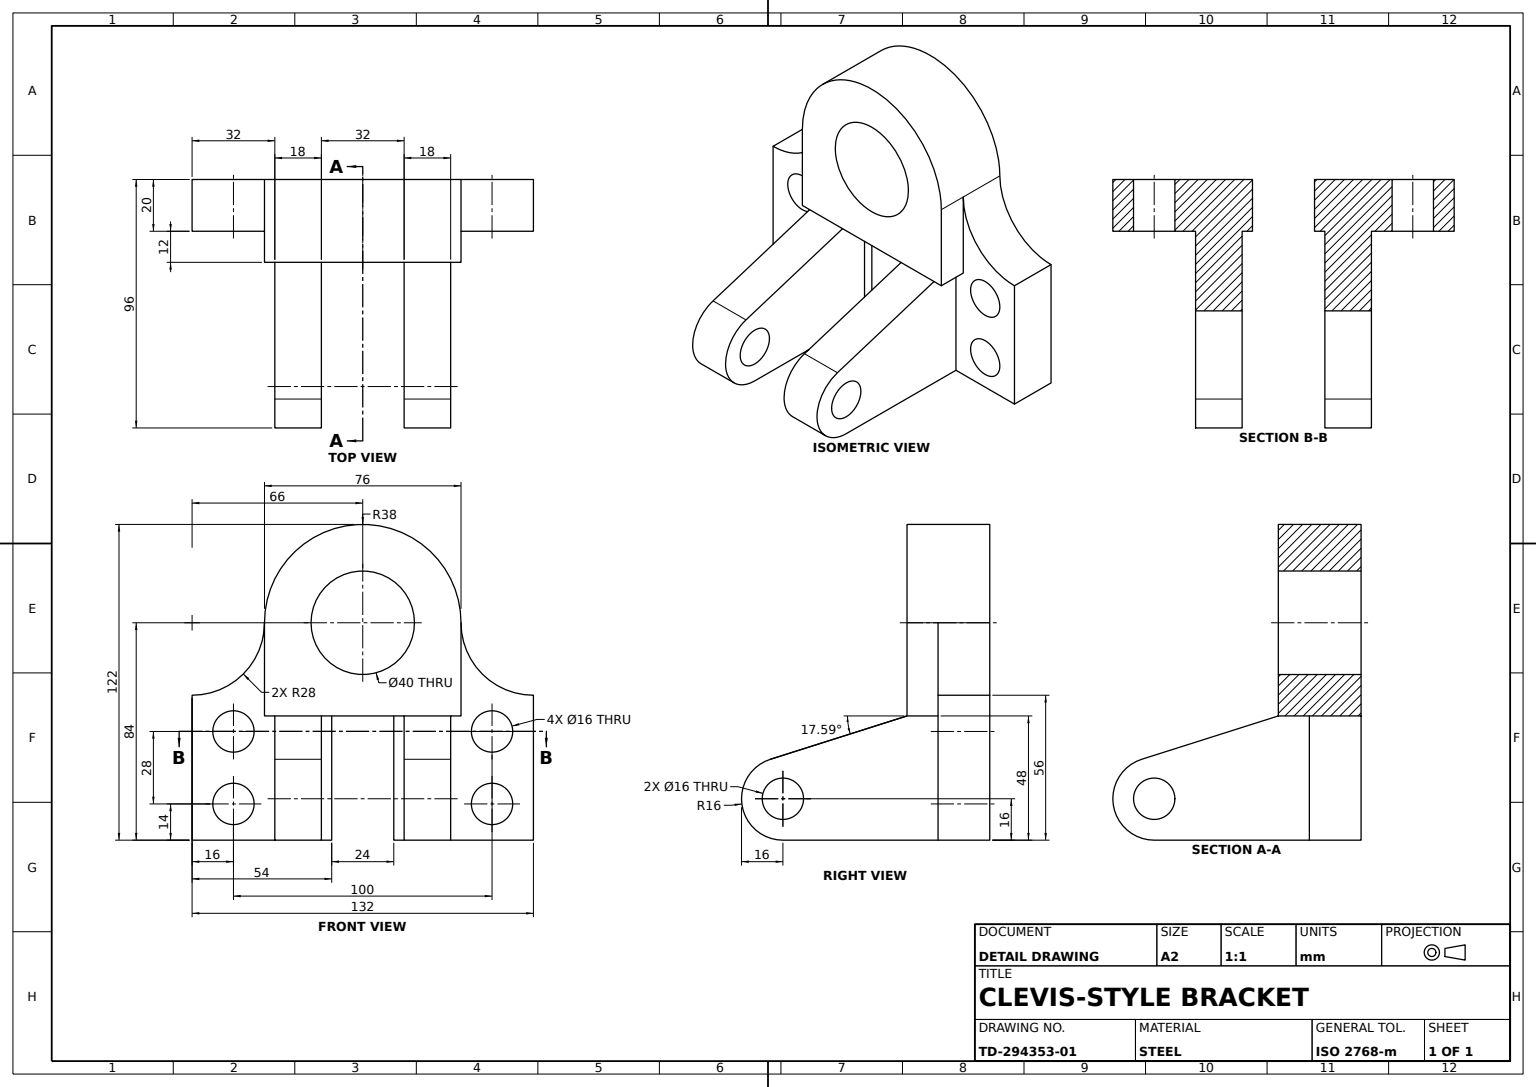
from build123d import *

# Parameters (mm, degrees)
BASE_PLATE_SKETCH_W       = 54
BASE_PLATE_SKETCH_H       = 84
BASE_PLATE_SKETCH_R       = 8
BASE_PLATE_DEPTH          = 20
BASE_PLATE_2_DEPTH        = 20
BEARING_BOSS_SKETCH_R     = 20
BEARING_BOSS_DEPTH        = 32
BORE_START                = -32
BORE_SKETCH_R             = 20
BORE_40_DEPTH             = 32
SIDE_CUT_DEPTH            = 32
CLEVIS_LUG_SKETCH_W       = 18
CLEVIS_LUG_SKETCH_H       = 48
CLEVIS_LUG_DEPTH          = 76
LUG_END_PROFILE_SKETCH_R  = 8
LUG_END_PROFILE_CUT_DEPTH = 76


with BuildPart() as part:
    # Base Plate Sketch → Base Plate (new body)
    with BuildSketch(Plane.XY):
        with Locations((-39, 19.918699187)):
            Rectangle(BASE_PLATE_SKETCH_W, BASE_PLATE_SKETCH_H)
        with Locations((-50, 19.918699187)):
            Circle(BASE_PLATE_SKETCH_R, mode=Mode.SUBTRACT)
        with Locations((-50, -8.081300813)):
            Circle(BASE_PLATE_SKETCH_R, mode=Mode.SUBTRACT)
    extrude(amount=-BASE_PLATE_DEPTH)



with BuildPart() as body_2:
    # Base Plate Sketch → Base Plate 2 (new body)
    with BuildSketch(Plane.XY):
        with Locations((39, 19.918699187)):
            Rectangle(BASE_PLATE_SKETCH_W, BASE_PLATE_SKETCH_H)
        with Locations(Location((50, -8.081300813, 0), (0, 0, 180))):
            Circle(BASE_PLATE_SKETCH_R, mode=Mode.SUBTRACT)
        with Locations(Location((50, 19.918699187, 0), (0, 0, 180))):
            Circle(BASE_PLATE_SKETCH_R, mode=Mode.SUBTRACT)
    extrude(amount=-BASE_PLATE_2_DEPTH)


with BuildPart() as part_1:
    add(part.part)

    add(body_2.part)  # Bearing Boss merges body 2
    # Bearing Boss Sketch → Bearing Boss (add)
    with BuildSketch(Plane(origin=(0, 0, -20), x_dir=(-1, 0, 0), z_dir=(0, 0, -1))):
        with BuildLine():
            Line((38, 61.918699187), (38, 25.918699187))
            Line((38, 25.918699187), (-38, 25.918699187))
            Line((-38, 25.918699187), (-38, 61.918699187))
            ThreePointArc((-38, 61.918699187), (0, 99.918699187), (38, 61.918699187))
        make_face()
        with Locations((0, 61.918699187)):
            Circle(BEARING_BOSS_SKETCH_R, mode=Mode.SUBTRACT)
    extrude(amount=-BEARING_BOSS_DEPTH)

    # Bore Sketch → Bore Ø40 (cut)
    with BuildSketch(Plane.XY.offset(12).offset(BORE_START)):
        with Locations(Location((0, 61.918699187, 0), (0, 0, 180))):
            Circle(BORE_SKETCH_R)
    extrude(amount=BORE_40_DEPTH, mode=Mode.SUBTRACT)

    # Side Cut Sketch → Side Cut (cut)
    with BuildSketch(Plane.XY):
        with BuildLine():
            ThreePointArc((-66, 33.918699187), (-46.201010127, 42.119709314), (-38, 61.918699187))
            Line((-38, 61.918699187), (-66, 61.918699187))
            Line((-66, 61.918699187), (-66, 33.918699187))
        make_face()
    side_cut = extrude(amount=-SIDE_CUT_DEPTH, mode=Mode.SUBTRACT)

    # Side Cut Mirror: Side Cut across plane
    add(side_cut.mirror(Plane(origin=(0, 0, 0), x_dir=(0, 0, 1), z_dir=(1, 0, 0))), mode=Mode.SUBTRACT)

    # Clevis Lug Sketch → Clevis Lug (add)
    with BuildSketch(Plane.XY):
        with Locations((-25, 1.918699187)):
            Rectangle(CLEVIS_LUG_SKETCH_W, CLEVIS_LUG_SKETCH_H)
    clevis_lug = extrude(amount=CLEVIS_LUG_DEPTH)

    # Clevis Lug Mirror: Clevis Lug across plane
    add(clevis_lug.mirror(Plane(origin=(0, 0, 0), x_dir=(0, 0, 1), z_dir=(1, 0, 0))))

    # Lug End Profile Sketch → Lug End Profile Cut (cut)
    with BuildSketch(Plane.ZY.offset(34)):
        with BuildLine():
            Line((76, 25.918699187), (12, 25.918699187))
            Line((12, 25.918699187), (64.834711668, 9.170766689))
            ThreePointArc((64.834711668, 9.170766689), (72.910371542, 3.3697471), (76, -6.081300813))
            Line((76, -6.081300813), (76, 25.918699187))
        make_face()
        with BuildLine():
            Line((76, -22.081300813), (76, -6.081300813))
            ThreePointArc((76, -6.081300813), (71.313708499, -17.395009312), (60, -22.081300813))
            Line((60, -22.081300813), (76, -22.081300813))
        make_face()
        with Locations((60, -6.081300813)):
            Circle(LUG_END_PROFILE_SKETCH_R)
    extrude(amount=-LUG_END_PROFILE_CUT_DEPTH, mode=Mode.SUBTRACT)


solid = part_1.part
